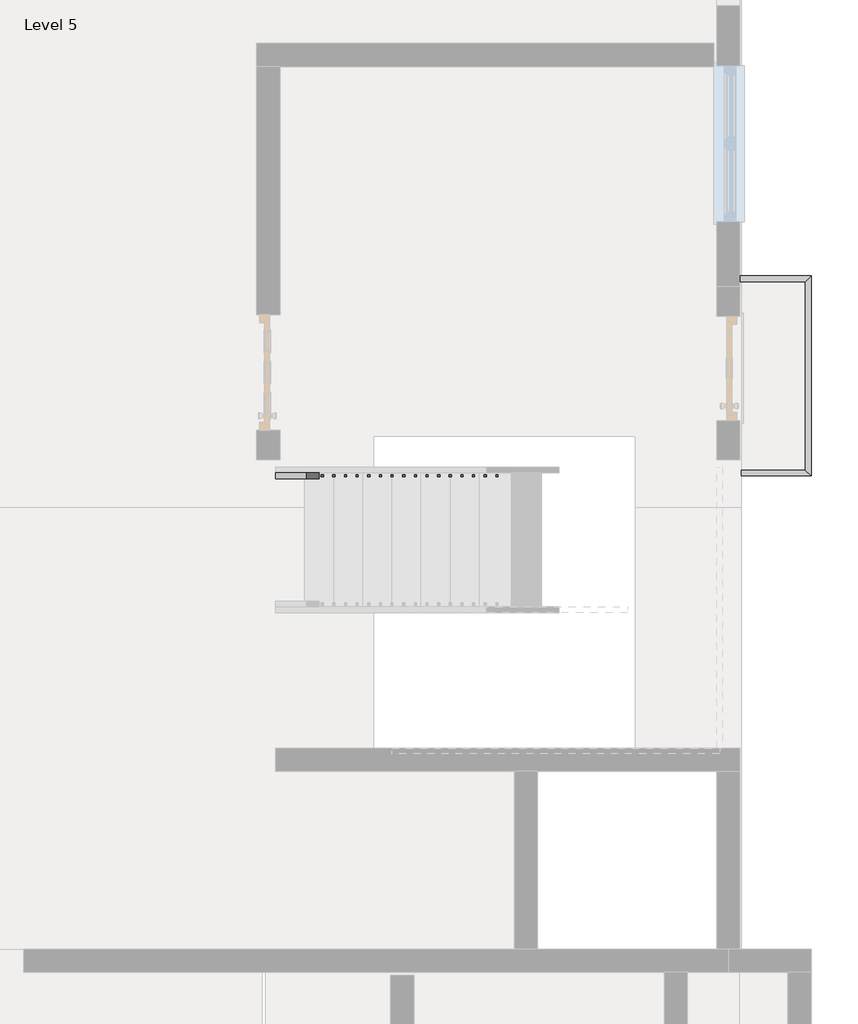
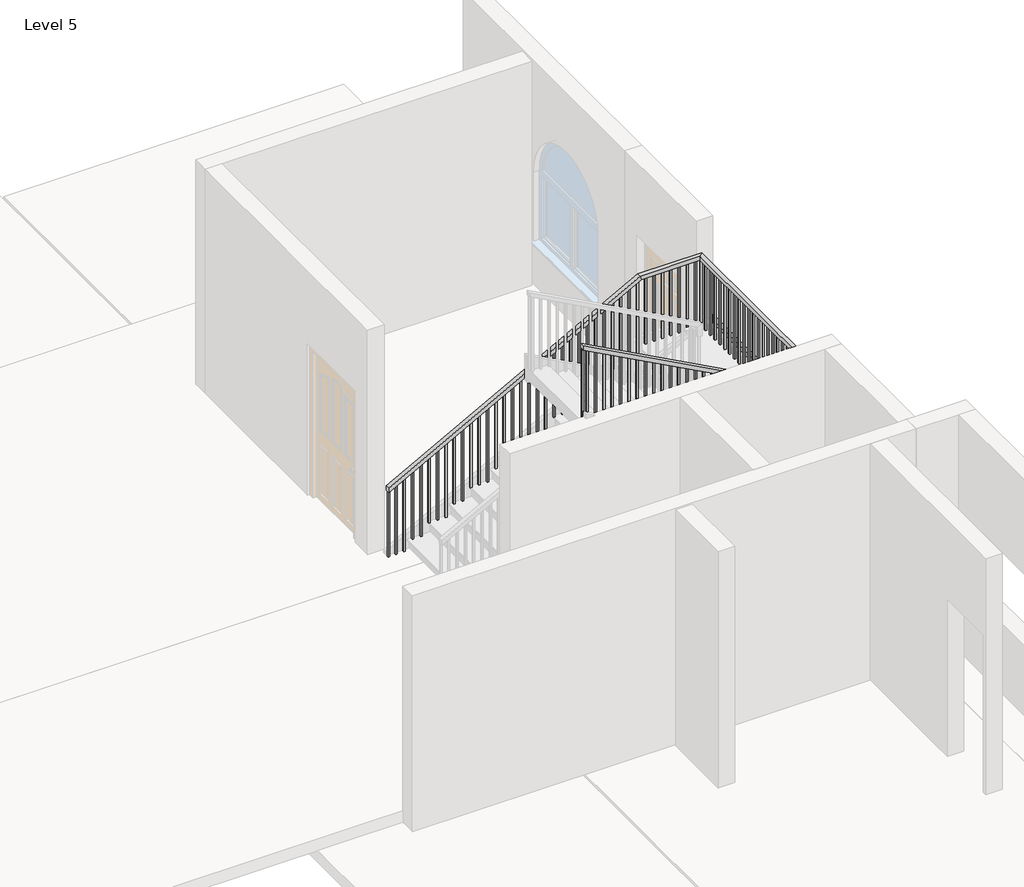
# One storey, part 6 of 7: 2 railings.
"""IFC4 building model written with IfcOpenShell, lengths in millimetres."""

from ifc_helpers import new_model, si_unit, frame, origin, place, context, project, spatial, polyline, outline, extrude, faceted_brep, element, save

model = new_model("IFC4")

# Units and contexts
model_context = context("Model", 3, world=origin())
ifc_project = project(units=[si_unit("LENGTHUNIT", "METRE", prefix="MILLI")], contexts=[model_context])

# Site, building, storey
site = spatial("IfcSite", under=ifc_project)
building = spatial("IfcBuilding", under=site)
storey = spatial("IfcBuildingStorey", under=building, Name="Level 5", Elevation=12192.0)

# Railings
placement = place(None, origin())
element("IfcRailing", 1, ObjectType="Handrail - Rectangular", at=placement, inside=storey, context=model_context, shape_type="SolidModel", body=[
    faceted_brep([(5863.1890963, 3183.81308, 13106.4), (5863.1890963, 3183.81308, 13055.6), (5863.1890963, 3133.01308, 13055.6), (5863.1890963, 3133.01308, 13106.4), (6485.4890963, 3183.81308, 13106.4), (6485.4890963, 3183.81308, 13055.6), (6434.6890963, 3133.01308, 13055.6), (6434.6890963, 3133.01308, 13106.4), (6485.4890963, 1439.3962251, 13106.4), (6485.4890963, 1439.3962251, 13055.6), (6434.6890963, 1490.1962251, 13055.6), (6434.6890963, 1490.1962251, 13106.4), (5875.8890963, 1439.3962251, 13106.4), (5875.8890963, 1490.1962251, 13106.4), (5875.8890963, 1490.1962251, 13055.6), (5875.8890963, 1439.3962251, 13055.6)], [[[0, 1, 2, 3]], [[1, 0, 4, 5]], [[2, 1, 5, 6]], [[3, 2, 6, 7]], [[0, 3, 7, 4]], [[5, 4, 8, 9]], [[6, 5, 9, 10]], [[7, 6, 10, 11]], [[4, 7, 11, 8]], [[12, 13, 14, 15]], [[9, 8, 12, 15]], [[10, 9, 15, 14]], [[11, 10, 14, 13]], [[8, 11, 13, 12]]]),
    extrude(outline(polyline([(5961.6140963, 1474.3212251), (5961.6140963, 1455.2712251), (5942.5640963, 1455.2712251), (5942.5640963, 1474.3212251), (5961.6140963, 1474.3212251)])), frame((0.0, 0.0, 12192.0), z_axis=(0.0, 0.0, 1.0), x_axis=(1.0, 0.0, 0.0)), (0.0, 0.0, 1.0), 863.6),
    extrude(outline(polyline([(6063.2140963, 1474.3212251), (6063.2140963, 1455.2712251), (6044.1640963, 1455.2712251), (6044.1640963, 1474.3212251), (6063.2140963, 1474.3212251)])), frame((0.0, 0.0, 12192.0), z_axis=(0.0, 0.0, 1.0), x_axis=(1.0, 0.0, 0.0)), (0.0, 0.0, 1.0), 863.6),
    extrude(outline(polyline([(6164.8140963, 1474.3212251), (6164.8140963, 1455.2712251), (6145.7640963, 1455.2712251), (6145.7640963, 1474.3212251), (6164.8140963, 1474.3212251)])), frame((0.0, 0.0, 12192.0), z_axis=(0.0, 0.0, 1.0), x_axis=(1.0, 0.0, 0.0)), (0.0, 0.0, 1.0), 863.6),
    extrude(outline(polyline([(6266.4140963, 1474.3212251), (6266.4140963, 1455.2712251), (6247.3640963, 1455.2712251), (6247.3640963, 1474.3212251), (6266.4140963, 1474.3212251)])), frame((0.0, 0.0, 12192.0), z_axis=(0.0, 0.0, 1.0), x_axis=(1.0, 0.0, 0.0)), (0.0, 0.0, 1.0), 863.6),
    extrude(outline(polyline([(6368.0140963, 1474.3212251), (6368.0140963, 1455.2712251), (6348.9640963, 1455.2712251), (6348.9640963, 1474.3212251), (6368.0140963, 1474.3212251)])), frame((0.0, 0.0, 12192.0), z_axis=(0.0, 0.0, 1.0), x_axis=(1.0, 0.0, 0.0)), (0.0, 0.0, 1.0), 863.6),
    extrude(outline(polyline([(6450.5640963, 1542.33808), (6469.6140963, 1542.33808), (6469.6140963, 1523.28808), (6450.5640963, 1523.28808), (6450.5640963, 1542.33808)])), frame((0.0, 0.0, 12192.0), z_axis=(0.0, 0.0, 1.0), x_axis=(1.0, 0.0, 0.0)), (0.0, 0.0, 1.0), 863.6),
    extrude(outline(polyline([(6450.5640963, 1643.93808), (6469.6140963, 1643.93808), (6469.6140963, 1624.88808), (6450.5640963, 1624.88808), (6450.5640963, 1643.93808)])), frame((0.0, 0.0, 12192.0), z_axis=(0.0, 0.0, 1.0), x_axis=(1.0, 0.0, 0.0)), (0.0, 0.0, 1.0), 863.6),
    extrude(outline(polyline([(6450.5640963, 1745.53808), (6469.6140963, 1745.53808), (6469.6140963, 1726.48808), (6450.5640963, 1726.48808), (6450.5640963, 1745.53808)])), frame((0.0, 0.0, 12192.0), z_axis=(0.0, 0.0, 1.0), x_axis=(1.0, 0.0, 0.0)), (0.0, 0.0, 1.0), 863.6),
    extrude(outline(polyline([(6450.5640963, 1847.13808), (6469.6140963, 1847.13808), (6469.6140963, 1828.08808), (6450.5640963, 1828.08808), (6450.5640963, 1847.13808)])), frame((0.0, 0.0, 12192.0), z_axis=(0.0, 0.0, 1.0), x_axis=(1.0, 0.0, 0.0)), (0.0, 0.0, 1.0), 863.6),
    extrude(outline(polyline([(6450.5640963, 1948.73808), (6469.6140963, 1948.73808), (6469.6140963, 1929.68808), (6450.5640963, 1929.68808), (6450.5640963, 1948.73808)])), frame((0.0, 0.0, 12192.0), z_axis=(0.0, 0.0, 1.0), x_axis=(1.0, 0.0, 0.0)), (0.0, 0.0, 1.0), 863.6),
    extrude(outline(polyline([(6450.5640963, 2050.33808), (6469.6140963, 2050.33808), (6469.6140963, 2031.28808), (6450.5640963, 2031.28808), (6450.5640963, 2050.33808)])), frame((0.0, 0.0, 12192.0), z_axis=(0.0, 0.0, 1.0), x_axis=(1.0, 0.0, 0.0)), (0.0, 0.0, 1.0), 863.6),
    extrude(outline(polyline([(6450.5640963, 2151.93808), (6469.6140963, 2151.93808), (6469.6140963, 2132.88808), (6450.5640963, 2132.88808), (6450.5640963, 2151.93808)])), frame((0.0, 0.0, 12192.0), z_axis=(0.0, 0.0, 1.0), x_axis=(1.0, 0.0, 0.0)), (0.0, 0.0, 1.0), 863.6),
    extrude(outline(polyline([(6450.5640963, 2253.53808), (6469.6140963, 2253.53808), (6469.6140963, 2234.48808), (6450.5640963, 2234.48808), (6450.5640963, 2253.53808)])), frame((0.0, 0.0, 12192.0), z_axis=(0.0, 0.0, 1.0), x_axis=(1.0, 0.0, 0.0)), (0.0, 0.0, 1.0), 863.6),
    extrude(outline(polyline([(6450.5640963, 2355.13808), (6469.6140963, 2355.13808), (6469.6140963, 2336.08808), (6450.5640963, 2336.08808), (6450.5640963, 2355.13808)])), frame((0.0, 0.0, 12192.0), z_axis=(0.0, 0.0, 1.0), x_axis=(1.0, 0.0, 0.0)), (0.0, 0.0, 1.0), 863.6),
    extrude(outline(polyline([(6450.5640963, 2456.73808), (6469.6140963, 2456.73808), (6469.6140963, 2437.68808), (6450.5640963, 2437.68808), (6450.5640963, 2456.73808)])), frame((0.0, 0.0, 12192.0), z_axis=(0.0, 0.0, 1.0), x_axis=(1.0, 0.0, 0.0)), (0.0, 0.0, 1.0), 863.6),
    extrude(outline(polyline([(6450.5640963, 2558.33808), (6469.6140963, 2558.33808), (6469.6140963, 2539.28808), (6450.5640963, 2539.28808), (6450.5640963, 2558.33808)])), frame((0.0, 0.0, 12192.0), z_axis=(0.0, 0.0, 1.0), x_axis=(1.0, 0.0, 0.0)), (0.0, 0.0, 1.0), 863.6),
    extrude(outline(polyline([(6450.5640963, 2659.93808), (6469.6140963, 2659.93808), (6469.6140963, 2640.88808), (6450.5640963, 2640.88808), (6450.5640963, 2659.93808)])), frame((0.0, 0.0, 12192.0), z_axis=(0.0, 0.0, 1.0), x_axis=(1.0, 0.0, 0.0)), (0.0, 0.0, 1.0), 863.6),
    extrude(outline(polyline([(6450.5640963, 2761.53808), (6469.6140963, 2761.53808), (6469.6140963, 2742.48808), (6450.5640963, 2742.48808), (6450.5640963, 2761.53808)])), frame((0.0, 0.0, 12192.0), z_axis=(0.0, 0.0, 1.0), x_axis=(1.0, 0.0, 0.0)), (0.0, 0.0, 1.0), 863.6),
    extrude(outline(polyline([(6450.5640963, 2863.13808), (6469.6140963, 2863.13808), (6469.6140963, 2844.08808), (6450.5640963, 2844.08808), (6450.5640963, 2863.13808)])), frame((0.0, 0.0, 12192.0), z_axis=(0.0, 0.0, 1.0), x_axis=(1.0, 0.0, 0.0)), (0.0, 0.0, 1.0), 863.6),
    extrude(outline(polyline([(6450.5640963, 2964.73808), (6469.6140963, 2964.73808), (6469.6140963, 2945.68808), (6450.5640963, 2945.68808), (6450.5640963, 2964.73808)])), frame((0.0, 0.0, 12192.0), z_axis=(0.0, 0.0, 1.0), x_axis=(1.0, 0.0, 0.0)), (0.0, 0.0, 1.0), 863.6),
    extrude(outline(polyline([(6450.5640963, 3066.33808), (6469.6140963, 3066.33808), (6469.6140963, 3047.28808), (6450.5640963, 3047.28808), (6450.5640963, 3066.33808)])), frame((0.0, 0.0, 12192.0), z_axis=(0.0, 0.0, 1.0), x_axis=(1.0, 0.0, 0.0)), (0.0, 0.0, 1.0), 863.6),
    extrude(outline(polyline([(6361.6640963, 3148.88808), (6361.6640963, 3167.93808), (6380.7140963, 3167.93808), (6380.7140963, 3148.88808), (6361.6640963, 3148.88808)])), frame((0.0, 0.0, 12192.0), z_axis=(0.0, 0.0, 1.0), x_axis=(1.0, 0.0, 0.0)), (0.0, 0.0, 1.0), 863.6),
    extrude(outline(polyline([(6260.0640963, 3148.88808), (6260.0640963, 3167.93808), (6279.1140963, 3167.93808), (6279.1140963, 3148.88808), (6260.0640963, 3148.88808)])), frame((0.0, 0.0, 12192.0), z_axis=(0.0, 0.0, 1.0), x_axis=(1.0, 0.0, 0.0)), (0.0, 0.0, 1.0), 863.6),
    extrude(outline(polyline([(6158.4640963, 3148.88808), (6158.4640963, 3167.93808), (6177.5140963, 3167.93808), (6177.5140963, 3148.88808), (6158.4640963, 3148.88808)])), frame((0.0, 0.0, 12192.0), z_axis=(0.0, 0.0, 1.0), x_axis=(1.0, 0.0, 0.0)), (0.0, 0.0, 1.0), 863.6),
    extrude(outline(polyline([(6056.8640963, 3148.88808), (6056.8640963, 3167.93808), (6075.9140963, 3167.93808), (6075.9140963, 3148.88808), (6056.8640963, 3148.88808)])), frame((0.0, 0.0, 12192.0), z_axis=(0.0, 0.0, 1.0), x_axis=(1.0, 0.0, 0.0)), (0.0, 0.0, 1.0), 863.6),
    extrude(outline(polyline([(5955.2640963, 3148.88808), (5955.2640963, 3167.93808), (5974.3140963, 3167.93808), (5974.3140963, 3148.88808), (5955.2640963, 3148.88808)])), frame((0.0, 0.0, 12192.0), z_axis=(0.0, 0.0, 1.0), x_axis=(1.0, 0.0, 0.0)), (0.0, 0.0, 1.0), 863.6),
    extrude(outline(polyline([(6450.5640963, 1474.3212251), (6469.6140963, 1474.3212251), (6469.6140963, 1455.2712251), (6450.5640963, 1455.2712251), (6450.5640963, 1474.3212251)])), frame((0.0, 0.0, 12192.0), z_axis=(0.0, 0.0, 1.0), x_axis=(1.0, 0.0, 0.0)), (0.0, 0.0, 1.0), 863.6),
    extrude(outline(polyline([(6450.5640963, 3148.88808), (6450.5640963, 3167.93808), (6469.6140963, 3167.93808), (6469.6140963, 3148.88808), (6450.5640963, 3148.88808)])), frame((0.0, 0.0, 12192.0), z_axis=(0.0, 0.0, 1.0), x_axis=(1.0, 0.0, 0.0)), (0.0, 0.0, 1.0), 863.6),
    extrude(outline(polyline([(5894.9390963, 1474.3212251), (5894.9390963, 1455.2712251), (5875.8890963, 1455.2712251), (5875.8890963, 1474.3212251), (5894.9390963, 1474.3212251)])), frame((0.0, 0.0, 12192.0), z_axis=(0.0, 0.0, 1.0), x_axis=(1.0, 0.0, 0.0)), (0.0, 0.0, 1.0), 863.6),
    extrude(outline(polyline([(5863.1890963, 3148.88808), (5863.1890963, 3167.93808), (5882.2390963, 3167.93808), (5882.2390963, 3148.88808), (5863.1890963, 3148.88808)])), frame((0.0, 0.0, 12192.0), z_axis=(0.0, 0.0, 1.0), x_axis=(1.0, 0.0, 0.0)), (0.0, 0.0, 1.0), 863.6),
])
element("IfcRailing", 2, ObjectType="Handrail - Rectangular", at=placement, inside=storey, context=model_context, shape_type="SolidModel", body=[
    faceted_brep([(1811.8890963, 1464.7962251, 13244.9454545), (1811.8890963, 1464.7962251, 13187.1709673), (1811.8890963, 1413.9962251, 13187.1709673), (1811.8890963, 1413.9962251, 13244.9454545), (4881.0326586, 1464.7962251, 14907.4909091), (4893.9079172, 1464.7962251, 14856.6909091), (4893.9079172, 1413.9962251, 14856.6909091), (4881.0326586, 1413.9962251, 14907.4909091), (5659.9890963, 1464.7962251, 14907.4909091), (5659.9890963, 1464.7962251, 14856.6909091), (5609.1890963, 1413.9962251, 14856.6909091), (5609.1890963, 1413.9962251, 14907.4909091), (5659.9890963, -935.5037749, 14907.4909091), (5659.9890963, -935.5037749, 14856.6909091), (5609.1890963, -884.7037749, 14856.6909091), (5609.1890963, -884.7037749, 14907.4909091), (5137.6756039, -935.5037749, 14907.4909091), (5124.8392301, -935.5037749, 14856.6909091), (5124.8392301, -884.7037749, 14856.6909091), (5137.6756039, -884.7037749, 14907.4909091), (2827.8890963, -935.5037749, 16154.4), (2827.8890963, -884.7037749, 16154.4), (2827.8890963, -884.7037749, 16096.6704456), (2827.8890963, -935.5037749, 16096.6704456)], [[[0, 1, 2, 3]], [[1, 0, 4, 5]], [[2, 1, 5, 6]], [[3, 2, 6, 7]], [[0, 3, 7, 4]], [[5, 4, 8, 9]], [[6, 5, 9, 10]], [[7, 6, 10, 11]], [[4, 7, 11, 8]], [[9, 8, 12, 13]], [[10, 9, 13, 14]], [[11, 10, 14, 15]], [[8, 11, 15, 12]], [[13, 12, 16, 17]], [[14, 13, 17, 18]], [[15, 14, 18, 19]], [[12, 15, 19, 16]], [[20, 21, 22, 23]], [[17, 16, 20, 23]], [[18, 17, 23, 22]], [[19, 18, 22, 21]], [[16, 19, 21, 20]]]),
    extrude(outline(polyline([(16067.5858236, 2881.8640963), (15101.4545455, 2881.8640963), (15101.4545455, 2900.9140963), (16057.2664983, 2900.9140963), (16067.5858236, 2881.8640963)])), frame((0.0, -919.6287749, 0.0), z_axis=(0.0, 1.0, 0.0), x_axis=(0.0, 0.0, 1.0)), (0.0, 0.0, 1.0), 19.05),
    extrude(outline(polyline([(16012.5494219, 2983.4640963), (15101.4545455, 2983.4640963), (15101.4545455, 3002.5140963), (16002.2300965, 3002.5140963), (16012.5494219, 2983.4640963)])), frame((0.0, -919.6287749, 0.0), z_axis=(0.0, 1.0, 0.0), x_axis=(0.0, 0.0, 1.0)), (0.0, 0.0, 1.0), 19.05),
    extrude(outline(polyline([(15957.8377681, 3085.0640963), (14962.9090909, 3085.0640963), (14962.9090909, 3104.1140963), (15947.553866, 3104.1140963), (15957.8377681, 3085.0640963)])), frame((0.0, -919.6287749, 0.0), z_axis=(0.0, 1.0, 0.0), x_axis=(0.0, 0.0, 1.0)), (0.0, 0.0, 1.0), 19.05),
    extrude(outline(polyline([(15902.9902905, 3186.6640963), (14962.9090909, 3186.6640963), (14962.9090909, 3205.7140963), (15892.7063885, 3205.7140963), (15902.9902905, 3186.6640963)])), frame((0.0, -919.6287749, 0.0), z_axis=(0.0, 1.0, 0.0), x_axis=(0.0, 0.0, 1.0)), (0.0, 0.0, 1.0), 19.05),
    extrude(outline(polyline([(15848.1428129, 3288.2640963), (14962.9090909, 3288.2640963), (14962.9090909, 3307.3140963), (15837.8589109, 3307.3140963), (15848.1428129, 3288.2640963)])), frame((0.0, -919.6287749, 0.0), z_axis=(0.0, 1.0, 0.0), x_axis=(0.0, 0.0, 1.0)), (0.0, 0.0, 1.0), 19.05),
    extrude(outline(polyline([(15793.2953354, 3389.8640963), (14824.3636364, 3389.8640963), (14824.3636364, 3408.9140963), (15783.0114333, 3408.9140963), (15793.2953354, 3389.8640963)])), frame((0.0, -919.6287749, 0.0), z_axis=(0.0, 1.0, 0.0), x_axis=(0.0, 0.0, 1.0)), (0.0, 0.0, 1.0), 19.05),
    extrude(outline(polyline([(15738.4478578, 3491.4640963), (14824.3636364, 3491.4640963), (14824.3636364, 3510.5140963), (15728.1639558, 3510.5140963), (15738.4478578, 3491.4640963)])), frame((0.0, -919.6287749, 0.0), z_axis=(0.0, 1.0, 0.0), x_axis=(0.0, 0.0, 1.0)), (0.0, 0.0, 1.0), 19.05),
    extrude(outline(polyline([(15683.6003803, 3593.0640963), (14685.8181818, 3593.0640963), (14685.8181818, 3612.1140963), (15673.3164782, 3612.1140963), (15683.6003803, 3593.0640963)])), frame((0.0, -919.6287749, 0.0), z_axis=(0.0, 1.0, 0.0), x_axis=(0.0, 0.0, 1.0)), (0.0, 0.0, 1.0), 19.05),
    extrude(outline(polyline([(15628.7529027, 3694.6640963), (14685.8181818, 3694.6640963), (14685.8181818, 3713.7140963), (15618.4690007, 3713.7140963), (15628.7529027, 3694.6640963)])), frame((0.0, -919.6287749, 0.0), z_axis=(0.0, 1.0, 0.0), x_axis=(0.0, 0.0, 1.0)), (0.0, 0.0, 1.0), 19.05),
    extrude(outline(polyline([(15573.9054252, 3796.2640963), (14685.8181818, 3796.2640963), (14685.8181818, 3815.3140963), (15563.6215231, 3815.3140963), (15573.9054252, 3796.2640963)])), frame((0.0, -919.6287749, 0.0), z_axis=(0.0, 1.0, 0.0), x_axis=(0.0, 0.0, 1.0)), (0.0, 0.0, 1.0), 19.05),
    extrude(outline(polyline([(15519.1307062, 3897.8640963), (14547.2727273, 3897.8640963), (14547.2727273, 3916.9140963), (15508.8113809, 3916.9140963), (15519.1307062, 3897.8640963)])), frame((0.0, -919.6287749, 0.0), z_axis=(0.0, 1.0, 0.0), x_axis=(0.0, 0.0, 1.0)), (0.0, 0.0, 1.0), 19.05),
    extrude(outline(polyline([(15464.0943044, 3999.4640963), (14547.2727273, 3999.4640963), (14547.2727273, 4018.5140963), (15453.7749791, 4018.5140963), (15464.0943044, 3999.4640963)])), frame((0.0, -919.6287749, 0.0), z_axis=(0.0, 1.0, 0.0), x_axis=(0.0, 0.0, 1.0)), (0.0, 0.0, 1.0), 19.05),
    extrude(outline(polyline([(15409.3629925, 4101.0640963), (14408.7272727, 4101.0640963), (14408.7272727, 4120.1140963), (15399.0790904, 4120.1140963), (15409.3629925, 4101.0640963)])), frame((0.0, -919.6287749, 0.0), z_axis=(0.0, 1.0, 0.0), x_axis=(0.0, 0.0, 1.0)), (0.0, 0.0, 1.0), 19.05),
    extrude(outline(polyline([(15354.5155149, 4202.6640963), (14408.7272727, 4202.6640963), (14408.7272727, 4221.7140963), (15344.2316129, 4221.7140963), (15354.5155149, 4202.6640963)])), frame((0.0, -919.6287749, 0.0), z_axis=(0.0, 1.0, 0.0), x_axis=(0.0, 0.0, 1.0)), (0.0, 0.0, 1.0), 19.05),
    extrude(outline(polyline([(15299.6680374, 4304.2640963), (14408.7272727, 4304.2640963), (14408.7272727, 4323.3140963), (15289.3841353, 4323.3140963), (15299.6680374, 4304.2640963)])), frame((0.0, -919.6287749, 0.0), z_axis=(0.0, 1.0, 0.0), x_axis=(0.0, 0.0, 1.0)), (0.0, 0.0, 1.0), 19.05),
    extrude(outline(polyline([(15244.8205598, 4405.8640963), (14270.1818182, 4405.8640963), (14270.1818182, 4424.9140963), (15234.5366578, 4424.9140963), (15244.8205598, 4405.8640963)])), frame((0.0, -919.6287749, 0.0), z_axis=(0.0, 1.0, 0.0), x_axis=(0.0, 0.0, 1.0)), (0.0, 0.0, 1.0), 19.05),
    extrude(outline(polyline([(15189.9730823, 4507.4640963), (14270.1818182, 4507.4640963), (14270.1818182, 4526.5140963), (15179.6891802, 4526.5140963), (15189.9730823, 4507.4640963)])), frame((0.0, -919.6287749, 0.0), z_axis=(0.0, 1.0, 0.0), x_axis=(0.0, 0.0, 1.0)), (0.0, 0.0, 1.0), 19.05),
    extrude(outline(polyline([(15135.1256047, 4609.0640963), (14131.6363636, 4609.0640963), (14131.6363636, 4628.1140963), (15124.8417027, 4628.1140963), (15135.1256047, 4609.0640963)])), frame((0.0, -919.6287749, 0.0), z_axis=(0.0, 1.0, 0.0), x_axis=(0.0, 0.0, 1.0)), (0.0, 0.0, 1.0), 19.05),
    extrude(outline(polyline([(15080.2781272, 4710.6640963), (14131.6363636, 4710.6640963), (14131.6363636, 4729.7140963), (15069.9942251, 4729.7140963), (15080.2781272, 4710.6640963)])), frame((0.0, -919.6287749, 0.0), z_axis=(0.0, 1.0, 0.0), x_axis=(0.0, 0.0, 1.0)), (0.0, 0.0, 1.0), 19.05),
    extrude(outline(polyline([(15025.4306496, 4812.2640963), (14131.6363636, 4812.2640963), (14131.6363636, 4831.3140963), (15015.1467476, 4831.3140963), (15025.4306496, 4812.2640963)])), frame((0.0, -919.6287749, 0.0), z_axis=(0.0, 1.0, 0.0), x_axis=(0.0, 0.0, 1.0)), (0.0, 0.0, 1.0), 19.05),
    extrude(outline(polyline([(14970.583172, 4913.8640963), (13993.0909091, 4913.8640963), (13993.0909091, 4932.9140963), (14960.29927, 4932.9140963), (14970.583172, 4913.8640963)])), frame((0.0, -919.6287749, 0.0), z_axis=(0.0, 1.0, 0.0), x_axis=(0.0, 0.0, 1.0)), (0.0, 0.0, 1.0), 19.05),
    extrude(outline(polyline([(14915.7356945, 5015.4640963), (13993.0909091, 5015.4640963), (13993.0909091, 5034.5140963), (14905.4517924, 5034.5140963), (14915.7356945, 5015.4640963)])), frame((0.0, -919.6287749, 0.0), z_axis=(0.0, 1.0, 0.0), x_axis=(0.0, 0.0, 1.0)), (0.0, 0.0, 1.0), 19.05),
    extrude(outline(polyline([(14860.8882169, 5117.0640963), (13993.0909091, 5117.0640963), (13993.0909091, 5136.1140963), (14850.6043149, 5136.1140963), (14860.8882169, 5117.0640963)])), frame((0.0, -919.6287749, 0.0), z_axis=(0.0, 1.0, 0.0), x_axis=(0.0, 0.0, 1.0)), (0.0, 0.0, 1.0), 19.05),
    extrude(outline(polyline([(5237.7140963, -919.6287749), (5218.6640963, -919.6287749), (5218.6640963, -900.5787749), (5237.7140963, -900.5787749), (5237.7140963, -919.6287749)])), frame((0.0, 0.0, 13993.0909091), z_axis=(0.0, 0.0, 1.0), x_axis=(1.0, 0.0, 0.0)), (0.0, 0.0, 1.0), 863.6),
    extrude(outline(polyline([(5339.3140963, -919.6287749), (5320.2640963, -919.6287749), (5320.2640963, -900.5787749), (5339.3140963, -900.5787749), (5339.3140963, -919.6287749)])), frame((0.0, 0.0, 13993.0909091), z_axis=(0.0, 0.0, 1.0), x_axis=(1.0, 0.0, 0.0)), (0.0, 0.0, 1.0), 863.6),
    extrude(outline(polyline([(5440.9140963, -919.6287749), (5421.8640963, -919.6287749), (5421.8640963, -900.5787749), (5440.9140963, -900.5787749), (5440.9140963, -919.6287749)])), frame((0.0, 0.0, 13993.0909091), z_axis=(0.0, 0.0, 1.0), x_axis=(1.0, 0.0, 0.0)), (0.0, 0.0, 1.0), 863.6),
    extrude(outline(polyline([(5542.5140963, -919.6287749), (5523.4640963, -919.6287749), (5523.4640963, -900.5787749), (5542.5140963, -900.5787749), (5542.5140963, -919.6287749)])), frame((0.0, 0.0, 13993.0909091), z_axis=(0.0, 0.0, 1.0), x_axis=(1.0, 0.0, 0.0)), (0.0, 0.0, 1.0), 863.6),
    extrude(outline(polyline([(5644.1140963, -887.8787749), (5644.1140963, -906.9287749), (5625.0640963, -906.9287749), (5625.0640963, -887.8787749), (5644.1140963, -887.8787749)])), frame((0.0, 0.0, 13993.0909091), z_axis=(0.0, 0.0, 1.0), x_axis=(1.0, 0.0, 0.0)), (0.0, 0.0, 1.0), 863.6),
    extrude(outline(polyline([(5644.1140963, -786.2787749), (5644.1140963, -805.3287749), (5625.0640963, -805.3287749), (5625.0640963, -786.2787749), (5644.1140963, -786.2787749)])), frame((0.0, 0.0, 13993.0909091), z_axis=(0.0, 0.0, 1.0), x_axis=(1.0, 0.0, 0.0)), (0.0, 0.0, 1.0), 863.6),
    extrude(outline(polyline([(5644.1140963, -684.6787749), (5644.1140963, -703.7287749), (5625.0640963, -703.7287749), (5625.0640963, -684.6787749), (5644.1140963, -684.6787749)])), frame((0.0, 0.0, 13993.0909091), z_axis=(0.0, 0.0, 1.0), x_axis=(1.0, 0.0, 0.0)), (0.0, 0.0, 1.0), 863.6),
    extrude(outline(polyline([(5644.1140963, -583.0787749), (5644.1140963, -602.1287749), (5625.0640963, -602.1287749), (5625.0640963, -583.0787749), (5644.1140963, -583.0787749)])), frame((0.0, 0.0, 13993.0909091), z_axis=(0.0, 0.0, 1.0), x_axis=(1.0, 0.0, 0.0)), (0.0, 0.0, 1.0), 863.6),
    extrude(outline(polyline([(5644.1140963, -481.4787749), (5644.1140963, -500.5287749), (5625.0640963, -500.5287749), (5625.0640963, -481.4787749), (5644.1140963, -481.4787749)])), frame((0.0, 0.0, 13993.0909091), z_axis=(0.0, 0.0, 1.0), x_axis=(1.0, 0.0, 0.0)), (0.0, 0.0, 1.0), 863.6),
    extrude(outline(polyline([(5644.1140963, -379.8787749), (5644.1140963, -398.9287749), (5625.0640963, -398.9287749), (5625.0640963, -379.8787749), (5644.1140963, -379.8787749)])), frame((0.0, 0.0, 13993.0909091), z_axis=(0.0, 0.0, 1.0), x_axis=(1.0, 0.0, 0.0)), (0.0, 0.0, 1.0), 863.6),
    extrude(outline(polyline([(5644.1140963, -278.2787749), (5644.1140963, -297.3287749), (5625.0640963, -297.3287749), (5625.0640963, -278.2787749), (5644.1140963, -278.2787749)])), frame((0.0, 0.0, 13993.0909091), z_axis=(0.0, 0.0, 1.0), x_axis=(1.0, 0.0, 0.0)), (0.0, 0.0, 1.0), 863.6),
    extrude(outline(polyline([(5644.1140963, -176.6787749), (5644.1140963, -195.7287749), (5625.0640963, -195.7287749), (5625.0640963, -176.6787749), (5644.1140963, -176.6787749)])), frame((0.0, 0.0, 13993.0909091), z_axis=(0.0, 0.0, 1.0), x_axis=(1.0, 0.0, 0.0)), (0.0, 0.0, 1.0), 863.6),
    extrude(outline(polyline([(5644.1140963, -75.0787749), (5644.1140963, -94.1287749), (5625.0640963, -94.1287749), (5625.0640963, -75.0787749), (5644.1140963, -75.0787749)])), frame((0.0, 0.0, 13993.0909091), z_axis=(0.0, 0.0, 1.0), x_axis=(1.0, 0.0, 0.0)), (0.0, 0.0, 1.0), 863.6),
    extrude(outline(polyline([(5644.1140963, 26.5212251), (5644.1140963, 7.4712251), (5625.0640963, 7.4712251), (5625.0640963, 26.5212251), (5644.1140963, 26.5212251)])), frame((0.0, 0.0, 13993.0909091), z_axis=(0.0, 0.0, 1.0), x_axis=(1.0, 0.0, 0.0)), (0.0, 0.0, 1.0), 863.6),
    extrude(outline(polyline([(5644.1140963, 128.1212251), (5644.1140963, 109.0712251), (5625.0640963, 109.0712251), (5625.0640963, 128.1212251), (5644.1140963, 128.1212251)])), frame((0.0, 0.0, 13993.0909091), z_axis=(0.0, 0.0, 1.0), x_axis=(1.0, 0.0, 0.0)), (0.0, 0.0, 1.0), 863.6),
    extrude(outline(polyline([(5644.1140963, 229.7212251), (5644.1140963, 210.6712251), (5625.0640963, 210.6712251), (5625.0640963, 229.7212251), (5644.1140963, 229.7212251)])), frame((0.0, 0.0, 13993.0909091), z_axis=(0.0, 0.0, 1.0), x_axis=(1.0, 0.0, 0.0)), (0.0, 0.0, 1.0), 863.6),
    extrude(outline(polyline([(5644.1140963, 331.3212251), (5644.1140963, 312.2712251), (5625.0640963, 312.2712251), (5625.0640963, 331.3212251), (5644.1140963, 331.3212251)])), frame((0.0, 0.0, 13993.0909091), z_axis=(0.0, 0.0, 1.0), x_axis=(1.0, 0.0, 0.0)), (0.0, 0.0, 1.0), 863.6),
    extrude(outline(polyline([(5644.1140963, 432.9212251), (5644.1140963, 413.8712251), (5625.0640963, 413.8712251), (5625.0640963, 432.9212251), (5644.1140963, 432.9212251)])), frame((0.0, 0.0, 13993.0909091), z_axis=(0.0, 0.0, 1.0), x_axis=(1.0, 0.0, 0.0)), (0.0, 0.0, 1.0), 863.6),
    extrude(outline(polyline([(5644.1140963, 534.5212251), (5644.1140963, 515.4712251), (5625.0640963, 515.4712251), (5625.0640963, 534.5212251), (5644.1140963, 534.5212251)])), frame((0.0, 0.0, 13993.0909091), z_axis=(0.0, 0.0, 1.0), x_axis=(1.0, 0.0, 0.0)), (0.0, 0.0, 1.0), 863.6),
    extrude(outline(polyline([(5644.1140963, 636.1212251), (5644.1140963, 617.0712251), (5625.0640963, 617.0712251), (5625.0640963, 636.1212251), (5644.1140963, 636.1212251)])), frame((0.0, 0.0, 13993.0909091), z_axis=(0.0, 0.0, 1.0), x_axis=(1.0, 0.0, 0.0)), (0.0, 0.0, 1.0), 863.6),
    extrude(outline(polyline([(5644.1140963, 737.7212251), (5644.1140963, 718.6712251), (5625.0640963, 718.6712251), (5625.0640963, 737.7212251), (5644.1140963, 737.7212251)])), frame((0.0, 0.0, 13993.0909091), z_axis=(0.0, 0.0, 1.0), x_axis=(1.0, 0.0, 0.0)), (0.0, 0.0, 1.0), 863.6),
    extrude(outline(polyline([(5644.1140963, 839.3212251), (5644.1140963, 820.2712251), (5625.0640963, 820.2712251), (5625.0640963, 839.3212251), (5644.1140963, 839.3212251)])), frame((0.0, 0.0, 13993.0909091), z_axis=(0.0, 0.0, 1.0), x_axis=(1.0, 0.0, 0.0)), (0.0, 0.0, 1.0), 863.6),
    extrude(outline(polyline([(5644.1140963, 940.9212251), (5644.1140963, 921.8712251), (5625.0640963, 921.8712251), (5625.0640963, 940.9212251), (5644.1140963, 940.9212251)])), frame((0.0, 0.0, 13993.0909091), z_axis=(0.0, 0.0, 1.0), x_axis=(1.0, 0.0, 0.0)), (0.0, 0.0, 1.0), 863.6),
    extrude(outline(polyline([(5644.1140963, 1042.5212251), (5644.1140963, 1023.4712251), (5625.0640963, 1023.4712251), (5625.0640963, 1042.5212251), (5644.1140963, 1042.5212251)])), frame((0.0, 0.0, 13993.0909091), z_axis=(0.0, 0.0, 1.0), x_axis=(1.0, 0.0, 0.0)), (0.0, 0.0, 1.0), 863.6),
    extrude(outline(polyline([(5644.1140963, 1144.1212251), (5644.1140963, 1125.0712251), (5625.0640963, 1125.0712251), (5625.0640963, 1144.1212251), (5644.1140963, 1144.1212251)])), frame((0.0, 0.0, 13993.0909091), z_axis=(0.0, 0.0, 1.0), x_axis=(1.0, 0.0, 0.0)), (0.0, 0.0, 1.0), 863.6),
    extrude(outline(polyline([(5644.1140963, 1245.7212251), (5644.1140963, 1226.6712251), (5625.0640963, 1226.6712251), (5625.0640963, 1245.7212251), (5644.1140963, 1245.7212251)])), frame((0.0, 0.0, 13993.0909091), z_axis=(0.0, 0.0, 1.0), x_axis=(1.0, 0.0, 0.0)), (0.0, 0.0, 1.0), 863.6),
    extrude(outline(polyline([(5644.1140963, 1347.3212251), (5644.1140963, 1328.2712251), (5625.0640963, 1328.2712251), (5625.0640963, 1347.3212251), (5644.1140963, 1347.3212251)])), frame((0.0, 0.0, 13993.0909091), z_axis=(0.0, 0.0, 1.0), x_axis=(1.0, 0.0, 0.0)), (0.0, 0.0, 1.0), 863.6),
    extrude(outline(polyline([(5561.5640963, 1448.9212251), (5580.6140963, 1448.9212251), (5580.6140963, 1429.8712251), (5561.5640963, 1429.8712251), (5561.5640963, 1448.9212251)])), frame((0.0, 0.0, 13993.0909091), z_axis=(0.0, 0.0, 1.0), x_axis=(1.0, 0.0, 0.0)), (0.0, 0.0, 1.0), 863.6),
    extrude(outline(polyline([(5459.9640963, 1448.9212251), (5479.0140963, 1448.9212251), (5479.0140963, 1429.8712251), (5459.9640963, 1429.8712251), (5459.9640963, 1448.9212251)])), frame((0.0, 0.0, 13993.0909091), z_axis=(0.0, 0.0, 1.0), x_axis=(1.0, 0.0, 0.0)), (0.0, 0.0, 1.0), 863.6),
    extrude(outline(polyline([(5358.3640963, 1448.9212251), (5377.4140963, 1448.9212251), (5377.4140963, 1429.8712251), (5358.3640963, 1429.8712251), (5358.3640963, 1448.9212251)])), frame((0.0, 0.0, 13993.0909091), z_axis=(0.0, 0.0, 1.0), x_axis=(1.0, 0.0, 0.0)), (0.0, 0.0, 1.0), 863.6),
    extrude(outline(polyline([(5256.7640963, 1448.9212251), (5275.8140963, 1448.9212251), (5275.8140963, 1429.8712251), (5256.7640963, 1429.8712251), (5256.7640963, 1448.9212251)])), frame((0.0, 0.0, 13993.0909091), z_axis=(0.0, 0.0, 1.0), x_axis=(1.0, 0.0, 0.0)), (0.0, 0.0, 1.0), 863.6),
    extrude(outline(polyline([(5155.1640963, 1448.9212251), (5174.2140963, 1448.9212251), (5174.2140963, 1429.8712251), (5155.1640963, 1429.8712251), (5155.1640963, 1448.9212251)])), frame((0.0, 0.0, 13993.0909091), z_axis=(0.0, 0.0, 1.0), x_axis=(1.0, 0.0, 0.0)), (0.0, 0.0, 1.0), 863.6),
    extrude(outline(polyline([(5053.5640963, 1448.9212251), (5072.6140963, 1448.9212251), (5072.6140963, 1429.8712251), (5053.5640963, 1429.8712251), (5053.5640963, 1448.9212251)])), frame((0.0, 0.0, 13993.0909091), z_axis=(0.0, 0.0, 1.0), x_axis=(1.0, 0.0, 0.0)), (0.0, 0.0, 1.0), 863.6),
    extrude(outline(polyline([(4951.9640963, 1448.9212251), (4971.0140963, 1448.9212251), (4971.0140963, 1429.8712251), (4951.9640963, 1429.8712251), (4951.9640963, 1448.9212251)])), frame((0.0, 0.0, 13993.0909091), z_axis=(0.0, 0.0, 1.0), x_axis=(1.0, 0.0, 0.0)), (0.0, 0.0, 1.0), 863.6),
    extrude(outline(polyline([(14833.1033577, 4850.3640963), (13854.5454545, 4850.3640963), (13854.5454545, 4869.4140963), (14843.422683, 4869.4140963), (14833.1033577, 4850.3640963)])), frame((0.0, 1429.8712251, 0.0), z_axis=(0.0, 1.0, 0.0), x_axis=(0.0, 0.0, 1.0)), (0.0, 0.0, 1.0), 19.05),
    extrude(outline(polyline([(14778.0669559, 4748.7640963), (13854.5454545, 4748.7640963), (13854.5454545, 4767.8140963), (14788.3862812, 4767.8140963), (14778.0669559, 4748.7640963)])), frame((0.0, 1429.8712251, 0.0), z_axis=(0.0, 1.0, 0.0), x_axis=(0.0, 0.0, 1.0)), (0.0, 0.0, 1.0), 19.05),
    extrude(outline(polyline([(14723.0305541, 4647.1640963), (13854.5454545, 4647.1640963), (13854.5454545, 4666.2140963), (14733.3498795, 4666.2140963), (14723.0305541, 4647.1640963)])), frame((0.0, 1429.8712251, 0.0), z_axis=(0.0, 1.0, 0.0), x_axis=(0.0, 0.0, 1.0)), (0.0, 0.0, 1.0), 19.05),
    extrude(outline(polyline([(14667.9941524, 4545.5640963), (13716.0, 4545.5640963), (13716.0, 4564.6140963), (14678.3134777, 4564.6140963), (14667.9941524, 4545.5640963)])), frame((0.0, 1429.8712251, 0.0), z_axis=(0.0, 1.0, 0.0), x_axis=(0.0, 0.0, 1.0)), (0.0, 0.0, 1.0), 19.05),
    extrude(outline(polyline([(14612.9577506, 4443.9640963), (13716.0, 4443.9640963), (13716.0, 4463.0140963), (14623.2770759, 4463.0140963), (14612.9577506, 4443.9640963)])), frame((0.0, 1429.8712251, 0.0), z_axis=(0.0, 1.0, 0.0), x_axis=(0.0, 0.0, 1.0)), (0.0, 0.0, 1.0), 19.05),
    extrude(outline(polyline([(14557.9213488, 4342.3640963), (13716.0, 4342.3640963), (13716.0, 4361.4140963), (14568.2406742, 4361.4140963), (14557.9213488, 4342.3640963)])), frame((0.0, 1429.8712251, 0.0), z_axis=(0.0, 1.0, 0.0), x_axis=(0.0, 0.0, 1.0)), (0.0, 0.0, 1.0), 19.05),
    extrude(outline(polyline([(14502.8849471, 4240.7640963), (13577.4545455, 4240.7640963), (13577.4545455, 4259.8140963), (14513.2042724, 4259.8140963), (14502.8849471, 4240.7640963)])), frame((0.0, 1429.8712251, 0.0), z_axis=(0.0, 1.0, 0.0), x_axis=(0.0, 0.0, 1.0)), (0.0, 0.0, 1.0), 19.05),
    extrude(outline(polyline([(14447.8485453, 4139.1640963), (13577.4545455, 4139.1640963), (13577.4545455, 4158.2140963), (14458.1678706, 4158.2140963), (14447.8485453, 4139.1640963)])), frame((0.0, 1429.8712251, 0.0), z_axis=(0.0, 1.0, 0.0), x_axis=(0.0, 0.0, 1.0)), (0.0, 0.0, 1.0), 19.05),
    extrude(outline(polyline([(14392.8121435, 4037.5640963), (13438.9090909, 4037.5640963), (13438.9090909, 4056.6140963), (14403.1314688, 4056.6140963), (14392.8121435, 4037.5640963)])), frame((0.0, 1429.8712251, 0.0), z_axis=(0.0, 1.0, 0.0), x_axis=(0.0, 0.0, 1.0)), (0.0, 0.0, 1.0), 19.05),
    extrude(outline(polyline([(14337.7757417, 3935.9640963), (13438.9090909, 3935.9640963), (13438.9090909, 3955.0140963), (14348.0950671, 3955.0140963), (14337.7757417, 3935.9640963)])), frame((0.0, 1429.8712251, 0.0), z_axis=(0.0, 1.0, 0.0), x_axis=(0.0, 0.0, 1.0)), (0.0, 0.0, 1.0), 19.05),
    extrude(outline(polyline([(14282.73934, 3834.3640963), (13438.9090909, 3834.3640963), (13438.9090909, 3853.4140963), (14293.0586653, 3853.4140963), (14282.73934, 3834.3640963)])), frame((0.0, 1429.8712251, 0.0), z_axis=(0.0, 1.0, 0.0), x_axis=(0.0, 0.0, 1.0)), (0.0, 0.0, 1.0), 19.05),
    extrude(outline(polyline([(14227.7029382, 3732.7640963), (13300.3636364, 3732.7640963), (13300.3636364, 3751.8140963), (14238.0222635, 3751.8140963), (14227.7029382, 3732.7640963)])), frame((0.0, 1429.8712251, 0.0), z_axis=(0.0, 1.0, 0.0), x_axis=(0.0, 0.0, 1.0)), (0.0, 0.0, 1.0), 19.05),
    extrude(outline(polyline([(14172.6665364, 3631.1640963), (13300.3636364, 3631.1640963), (13300.3636364, 3650.2140963), (14182.9858618, 3650.2140963), (14172.6665364, 3631.1640963)])), frame((0.0, 1429.8712251, 0.0), z_axis=(0.0, 1.0, 0.0), x_axis=(0.0, 0.0, 1.0)), (0.0, 0.0, 1.0), 19.05),
    extrude(outline(polyline([(14117.6301347, 3529.5640963), (13161.8181818, 3529.5640963), (13161.8181818, 3548.6140963), (14127.94946, 3548.6140963), (14117.6301347, 3529.5640963)])), frame((0.0, 1429.8712251, 0.0), z_axis=(0.0, 1.0, 0.0), x_axis=(0.0, 0.0, 1.0)), (0.0, 0.0, 1.0), 19.05),
    extrude(outline(polyline([(14062.5937329, 3427.9640963), (13161.8181818, 3427.9640963), (13161.8181818, 3447.0140963), (14072.9130582, 3447.0140963), (14062.5937329, 3427.9640963)])), frame((0.0, 1429.8712251, 0.0), z_axis=(0.0, 1.0, 0.0), x_axis=(0.0, 0.0, 1.0)), (0.0, 0.0, 1.0), 19.05),
    extrude(outline(polyline([(14007.5573311, 3326.3640963), (13161.8181818, 3326.3640963), (13161.8181818, 3345.4140963), (14017.8766565, 3345.4140963), (14007.5573311, 3326.3640963)])), frame((0.0, 1429.8712251, 0.0), z_axis=(0.0, 1.0, 0.0), x_axis=(0.0, 0.0, 1.0)), (0.0, 0.0, 1.0), 19.05),
    extrude(outline(polyline([(13952.5209294, 3224.7640963), (13023.2727273, 3224.7640963), (13023.2727273, 3243.8140963), (13962.8402547, 3243.8140963), (13952.5209294, 3224.7640963)])), frame((0.0, 1429.8712251, 0.0), z_axis=(0.0, 1.0, 0.0), x_axis=(0.0, 0.0, 1.0)), (0.0, 0.0, 1.0), 19.05),
    extrude(outline(polyline([(13897.4845276, 3123.1640963), (13023.2727273, 3123.1640963), (13023.2727273, 3142.2140963), (13907.8038529, 3142.2140963), (13897.4845276, 3123.1640963)])), frame((0.0, 1429.8712251, 0.0), z_axis=(0.0, 1.0, 0.0), x_axis=(0.0, 0.0, 1.0)), (0.0, 0.0, 1.0), 19.05),
    extrude(outline(polyline([(13842.4481258, 3021.5640963), (12884.7272727, 3021.5640963), (12884.7272727, 3040.6140963), (13852.7674512, 3040.6140963), (13842.4481258, 3021.5640963)])), frame((0.0, 1429.8712251, 0.0), z_axis=(0.0, 1.0, 0.0), x_axis=(0.0, 0.0, 1.0)), (0.0, 0.0, 1.0), 19.05),
    extrude(outline(polyline([(13787.4117241, 2919.9640963), (12884.7272727, 2919.9640963), (12884.7272727, 2939.0140963), (13797.7310494, 2939.0140963), (13787.4117241, 2919.9640963)])), frame((0.0, 1429.8712251, 0.0), z_axis=(0.0, 1.0, 0.0), x_axis=(0.0, 0.0, 1.0)), (0.0, 0.0, 1.0), 19.05),
    extrude(outline(polyline([(13732.3753223, 2818.3640963), (12884.7272727, 2818.3640963), (12884.7272727, 2837.4140963), (13742.6946476, 2837.4140963), (13732.3753223, 2818.3640963)])), frame((0.0, 1429.8712251, 0.0), z_axis=(0.0, 1.0, 0.0), x_axis=(0.0, 0.0, 1.0)), (0.0, 0.0, 1.0), 19.05),
    extrude(outline(polyline([(13677.3389205, 2716.7640963), (12746.1818182, 2716.7640963), (12746.1818182, 2735.8140963), (13687.6582459, 2735.8140963), (13677.3389205, 2716.7640963)])), frame((0.0, 1429.8712251, 0.0), z_axis=(0.0, 1.0, 0.0), x_axis=(0.0, 0.0, 1.0)), (0.0, 0.0, 1.0), 19.05),
    extrude(outline(polyline([(13622.3025188, 2615.1640963), (12746.1818182, 2615.1640963), (12746.1818182, 2634.2140963), (13632.6218441, 2634.2140963), (13622.3025188, 2615.1640963)])), frame((0.0, 1429.8712251, 0.0), z_axis=(0.0, 1.0, 0.0), x_axis=(0.0, 0.0, 1.0)), (0.0, 0.0, 1.0), 19.05),
    extrude(outline(polyline([(13567.266117, 2513.5640963), (12607.6363636, 2513.5640963), (12607.6363636, 2532.6140963), (13577.5854423, 2532.6140963), (13567.266117, 2513.5640963)])), frame((0.0, 1429.8712251, 0.0), z_axis=(0.0, 1.0, 0.0), x_axis=(0.0, 0.0, 1.0)), (0.0, 0.0, 1.0), 19.05),
    extrude(outline(polyline([(13512.2297152, 2411.9640963), (12607.6363636, 2411.9640963), (12607.6363636, 2431.0140963), (13522.5490405, 2431.0140963), (13512.2297152, 2411.9640963)])), frame((0.0, 1429.8712251, 0.0), z_axis=(0.0, 1.0, 0.0), x_axis=(0.0, 0.0, 1.0)), (0.0, 0.0, 1.0), 19.05),
    extrude(outline(polyline([(13457.1933134, 2310.3640963), (12607.6363636, 2310.3640963), (12607.6363636, 2329.4140963), (13467.5126388, 2329.4140963), (13457.1933134, 2310.3640963)])), frame((0.0, 1429.8712251, 0.0), z_axis=(0.0, 1.0, 0.0), x_axis=(0.0, 0.0, 1.0)), (0.0, 0.0, 1.0), 19.05),
    extrude(outline(polyline([(13402.1569117, 2208.7640963), (12469.0909091, 2208.7640963), (12469.0909091, 2227.8140963), (13412.476237, 2227.8140963), (13402.1569117, 2208.7640963)])), frame((0.0, 1429.8712251, 0.0), z_axis=(0.0, 1.0, 0.0), x_axis=(0.0, 0.0, 1.0)), (0.0, 0.0, 1.0), 19.05),
    extrude(outline(polyline([(13347.1205099, 2107.1640963), (12469.0909091, 2107.1640963), (12469.0909091, 2126.2140963), (13357.4398352, 2126.2140963), (13347.1205099, 2107.1640963)])), frame((0.0, 1429.8712251, 0.0), z_axis=(0.0, 1.0, 0.0), x_axis=(0.0, 0.0, 1.0)), (0.0, 0.0, 1.0), 19.05),
    extrude(outline(polyline([(13292.0841081, 2005.5640963), (12330.5454545, 2005.5640963), (12330.5454545, 2024.6140963), (13302.4034335, 2024.6140963), (13292.0841081, 2005.5640963)])), frame((0.0, 1429.8712251, 0.0), z_axis=(0.0, 1.0, 0.0), x_axis=(0.0, 0.0, 1.0)), (0.0, 0.0, 1.0), 19.05),
    extrude(outline(polyline([(13237.0477064, 1903.9640963), (12330.5454545, 1903.9640963), (12330.5454545, 1923.0140963), (13247.3670317, 1923.0140963), (13237.0477064, 1903.9640963)])), frame((0.0, 1429.8712251, 0.0), z_axis=(0.0, 1.0, 0.0), x_axis=(0.0, 0.0, 1.0)), (0.0, 0.0, 1.0), 19.05),
    extrude(outline(polyline([(5644.1140963, -900.5787749), (5644.1140963, -919.6287749), (5625.0640963, -919.6287749), (5625.0640963, -900.5787749), (5644.1140963, -900.5787749)])), frame((0.0, 0.0, 13993.0909091), z_axis=(0.0, 0.0, 1.0), x_axis=(1.0, 0.0, 0.0)), (0.0, 0.0, 1.0), 863.6),
    extrude(outline(polyline([(5625.0640963, 1448.9212251), (5644.1140963, 1448.9212251), (5644.1140963, 1429.8712251), (5625.0640963, 1429.8712251), (5625.0640963, 1448.9212251)])), frame((0.0, 0.0, 13993.0909091), z_axis=(0.0, 0.0, 1.0), x_axis=(1.0, 0.0, 0.0)), (0.0, 0.0, 1.0), 863.6),
    extrude(outline(polyline([(16096.6704456, 2827.8890963), (15101.4545455, 2827.8890963), (15101.4545455, 2846.9390963), (16086.3865436, 2846.9390963), (16096.6704456, 2827.8890963)])), frame((0.0, -919.6287749, 0.0), z_axis=(0.0, 1.0, 0.0), x_axis=(0.0, 0.0, 1.0)), (0.0, 0.0, 1.0), 19.05),
    extrude(outline(polyline([(13187.1709673, 1811.8890963), (12330.5454545, 1811.8890963), (12330.5454545, 1830.9390963), (13197.4902926, 1830.9390963), (13187.1709673, 1811.8890963)])), frame((0.0, 1429.8712251, 0.0), z_axis=(0.0, 1.0, 0.0), x_axis=(0.0, 0.0, 1.0)), (0.0, 0.0, 1.0), 19.05),
])

save(model, "model.ifc")

# Revit data of these elements
# Type "Handrail - Rectangular"
#   Assembly Code = "C2010400"
#   built-in parameter 1008612 = 0.0416667 (stored number, unit not read)
#   built-in parameter 1008611 = 0.0416667 (stored number, unit not read)
#   built-in parameter 1008609 = 0.333333 (stored number, unit not read)
#   built-in parameter 1008604 = 0.166667 (stored number, unit not read)
#   built-in parameter 1008603 = 0.166667 (stored number, unit not read)
#   Railing Height = 3' - 0"
#   built-in parameter 1008630 = 2
#   built-in parameter 1008610 = 2
#   built-in parameter 1008618 = Baluster - Square : 3/4"
# Elements 1, 2 (IfcRailing, "Handrail - Rectangular")
#   Phase Created = New Construction
